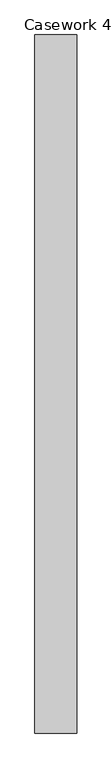
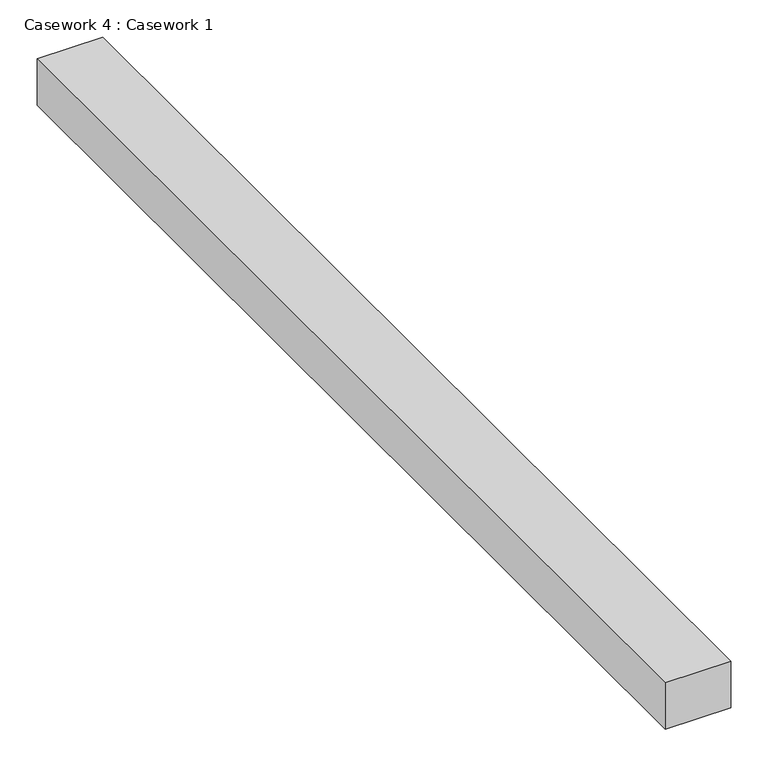
"""IFC4 building model written with IfcOpenShell, lengths in millimetres: furniture geometry, Casework 4 : Casework 1."""

from ifc_helpers import new_model, si_unit, frame, origin, place, context, project, spatial, polyline, outline, extrude, source, transform, mapped, element, save


def casework_4_casework_1_a5b175c9(model_context):
    return source(origin(), model_context, "Body", "SweptSolid", [
        extrude(outline(polyline([(8748.1559589, 14787.9496924), (8748.1559589, 13098.8496924), (8646.5559589, 13098.8496924), (8646.5559589, 14787.9496924), (8748.1559589, 14787.9496924)])), frame((0.0, 0.0, 3581.4), z_axis=(0.0, 0.0, 1.0), x_axis=(1.0, 0.0, 0.0)), (0.0, 0.0, 1.0), 76.2),
    ])


if __name__ == "__main__":
    model = new_model("IFC4")
    model_context = context("Model", 3, world=origin())
    ifc_project = project(units=[si_unit("LENGTHUNIT", "METRE", prefix="MILLI")], contexts=[model_context])
    site = spatial("IfcSite", under=ifc_project)
    building = spatial("IfcBuilding", under=site)
    placement = place(None, origin())
    casework_4_casework_1_shape = casework_4_casework_1_a5b175c9(model_context)
    element("IfcFurniture", 1, ObjectType="Casework 4 : Casework 1", at=placement, inside=building, context=model_context, shape_type="MappedRepresentation", body=[
        mapped(casework_4_casework_1_shape, transform((0.0, 0.0, 0.0), x_axis=(1.0, 0.0, 0.0), y_axis=(0.0, 1.0, 0.0), z_axis=(0.0, 0.0, 1.0))),
    ])
    save(model, "model.ifc")

# Revit data of these elements
# Element 1 (IfcFurniture, "Casework 4 : Casework 1")
#   Materials on its faces: "Clad - White"
# Materials
#   "Clad - White": class "Wood", colour RGB 242 242 238, transparency 0, Cost = 0
